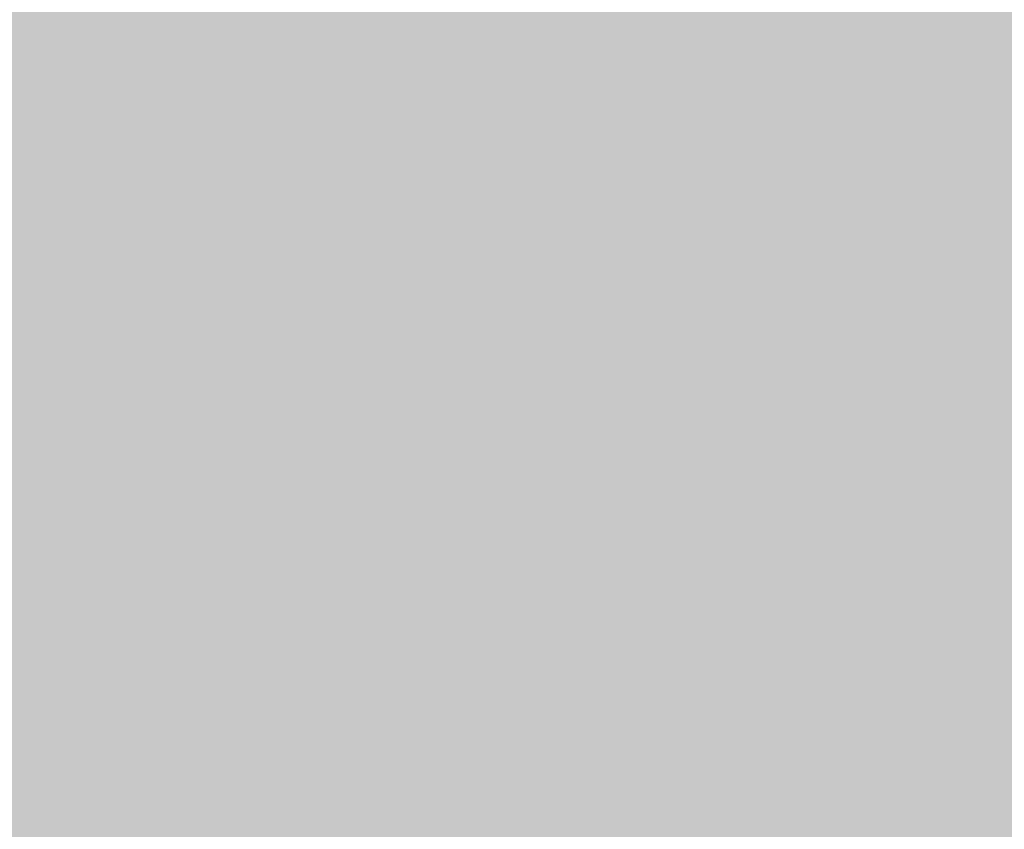
# Model space of a CAD drawing. Units: feet. Extents: x 3168 to 4724, y 827 to 1477.
# Tile 227 of 256: x 3379.08 to 3382.882, y 1093.654 to 1096.781. Entities that reach past the tile are written whole.
import ezdxf

# ---------------------------------------------------------------- set-up
doc = ezdxf.new("R2010")
doc.units = ezdxf.units.FT
doc.layers.add('A-ELEV-PATT', color=8, linetype='Continuous', lineweight=13)

msp = doc.modelspace()

# ---------------------------------------------------------------- hatches: boundary and pattern name
at = {"layer": 'A-ELEV-PATT'}
h = msp.add_hatch(color=256, dxfattribs=at)
h.dxf.hatch_style = 1
edge = h.paths.add_edge_path()
edge.add_ellipse((3552.9058, 979.2201), major_axis=(36.7449, 0), ratio=0.4848485, start_angle=0, end_angle=360)
edge = h.paths.add_edge_path()
edge.add_ellipse((3559.8916, 929.2523), major_axis=(36.7449, 0), ratio=0.4848485, start_angle=0, end_angle=360)
edge = h.paths.add_edge_path()
edge.add_line((3299.3168, 1198.6061), (3479.9167, 1198.6061))
edge.add_line((3479.9167, 1198.6061), (3479.9167, 1209.8686))
edge.add_spline(control_points=[(3479.9167, 1209.8686), (3464.3012, 1209.8686), (3448.6856, 1209.8686), (3410.9491, 1209.8686), (3388.8282, 1209.8686), (3355.6469, 1209.8686), (3344.5864, 1209.8686), (3327.9957, 1209.8686), (3322.4655, 1209.8686), (3314.1702, 1209.8686), (3311.4051, 1209.8686), (3307.2574, 1209.8686), (3305.8748, 1209.8686), (3303.801, 1209.8686), (3303.1097, 1209.8686), (3302.0728, 1209.8686), (3301.7272, 1209.8686), (3301.2087, 1209.8686), (3301.0359, 1209.8686), (3300.7767, 1209.8686), (3300.6903, 1209.8686), (3300.5606, 1209.8686), (3300.5174, 1209.8686), (3300.4526, 1209.8686), (3300.431, 1209.8686), (3300.3986, 1209.8686), (3300.3878, 1209.8686), (3300.3662, 1209.8686), (3300.3457, 1209.8686), (3300.3455, 1209.8686), (3300.3455, 1209.8686), (3300.3433, 1209.8686), (3300.3411, 1209.8686), (3300.3379, 1209.8686), (3300.3368, 1209.8686), (3300.3339, 1209.8686), (3300.3321, 1209.8686), (3300.3255, 1209.8686), (3300.3207, 1209.8686), (3300.3109, 1209.8686), (3300.306, 1209.8686), (3300.2905, 1209.8686), (3300.28, 1209.8686), (3300.2324, 1209.8688), (3300.1953, 1209.869), (3299.9511, 1209.8706), (3299.7448, 1209.8743), (3299.4368, 1209.8833), (3299.3344, 1209.8868), (3299.1811, 1209.8929), (3299.13, 1209.8951), (3298.6522, 1209.9168), (3298.2295, 1209.9457), (3297.6016, 1210.0024), (3297.3934, 1210.0235), (3297.0827, 1210.0583), (3296.9793, 1210.0705), (3296.293, 1210.1549), (3295.7181, 1210.2434), (3294.8687, 1210.3989), (3294.5877, 1210.4545), (3294.1693, 1210.5433), (3294.0304, 1210.5739), (3291.7071, 1211.1012), (3289.6536, 1211.8134), (3285.7763, 1213.564), (3283.9514, 1214.6035), (3280.5122, 1216.9801), (3278.8972, 1218.3176), (3276.3799, 1220.8295), (3275.416, 1221.9177), (3274.0393, 1223.7077), (3273.581, 1224.3495), (3273.1432, 1225.0163)], knot_values=[39.119033, 39.119033, 39.119033, 39.119033, 39.286353, 39.286353, 39.523379, 39.523379, 39.641892, 39.641892, 39.701148, 39.701148, 39.730777, 39.730777, 39.745591, 39.745591, 39.752998, 39.752998, 39.756701, 39.756701, 39.758553, 39.758553, 39.759479, 39.759479, 39.759942, 39.759942, 39.760173, 39.760173, 39.760289, 39.760289, 39.760405, 39.760405, 39.760463, 39.760463, 39.763389, 39.763389, 39.764851, 39.764851, 39.767304, 39.767304, 39.773825, 39.773825, 39.78057, 39.78057, 39.79477, 39.79477, 39.845194, 39.845194, 40.126715, 40.126715, 40.267476, 40.267476, 40.337856, 40.337856, 40.927023, 40.927023, 41.221606, 41.221606, 41.368898, 41.368898, 42.202622, 42.202622, 42.619485, 42.619485, 42.827916, 42.827916, 46.118323, 46.118323, 49.408731, 49.408731, 52.699139, 52.699139, 54.927489, 54.927489, 56.104228, 56.104228, 56.104228, 56.104228], weights=[1, 1, 1, 1, 1, 1, 1, 1, 1, 1, 1, 1, 1, 1, 1, 1, 1, 1, 1, 1, 1, 1, 1, 1, 1, 1, 1, 1, 1, 1, 1, 1, 1, 1, 1, 1, 1, 1, 1, 1, 1, 1, 1, 1, 1, 1, 1, 1, 1, 1, 1, 1, 1, 1, 1, 1, 1, 1, 1, 1, 1, 1, 1, 1, 1, 1, 1, 1, 1, 1, 1, 1, 1, 1], degree=3, periodic=0)
edge.add_line((3273.1432, 1225.0163), (3273.1432, 1099.0163))
edge.add_line((3273.1432, 1099.0163), (3299.3168, 1099.0163))
edge.add_line((3299.3168, 1099.0163), (3299.3168, 1198.6061))
edge = h.paths.add_edge_path()
edge.add_line((3304.7584, 1324.1581), (3479.9167, 1324.1581))
edge.add_line((3479.9167, 1324.1581), (3479.9167, 1335.7146))
edge.add_line((3479.9167, 1335.7146), (3269.1616, 1335.7146))
edge.add_spline(control_points=[(3269.1616, 1335.7146), (3264.0242, 1335.7146), (3258.3641, 1328.9582), (3259.2643, 1323.9003)], knot_values=[0, 0, 0, 0, 15.412191, 15.412191, 15.412191, 15.412191], degree=3, periodic=0)
edge.add_line((3259.2643, 1323.9003), (3265.5168, 1288.7691))
edge.add_line((3265.5168, 1288.7691), (3275.2651, 1261.5456))
edge.add_line((3275.2651, 1261.5456), (3304.7584, 1261.5456))
edge.add_line((3304.7584, 1261.5456), (3304.7584, 1324.1581))
h = msp.add_hatch(color=256, dxfattribs=at)
h.dxf.hatch_style = 1
h.paths.add_polyline_path([(3384.5252, 1099.0163), (3335.0292, 1099.0163), (3299.3168, 1099.0163), (3273.1432, 1099.0163), (3217.5654, 1099.0163), (3168.0693, 827.1163), (3335.0292, 827.1163)])

doc.saveas('drawing.dxf')
